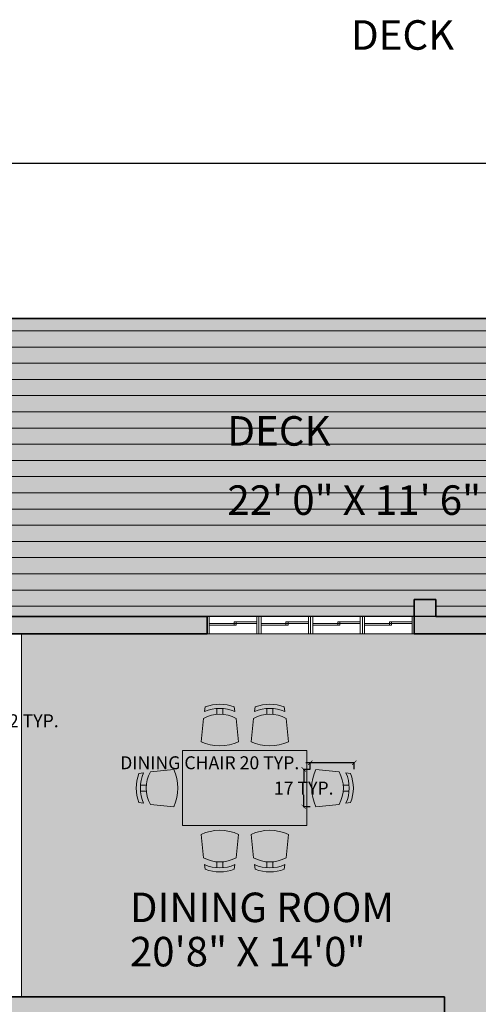
# Model space of a CAD drawing. Units: inches. Extents: x 1704 to 6393, y -157 to 1172.
# Tile 85 of 122: x 2081 to 2293, y 716 to 1172. Entities that reach past the tile are written whole.
import ezdxf

# ---------------------------------------------------------------- set-up
doc = ezdxf.new("R2010")
doc.units = ezdxf.units.IN
doc.header["$MEASUREMENT"] = 0
for name, color, linetype, lineweight in [('A-ANNO-DIMS', 7, 'Continuous', 13), ('A-AREA-IDEN', 7, 'Continuous', 18), ('A-FURN', 8, 'Continuous', 18), ('A-WALL-PATT', 7, 'Continuous', 13), ('C-PROP', 7, 'Continuous', 35), ('GLASS PANEL FASADE', 4, 'Continuous', 18), ('L-DECK-PLNK-PATT', 250, 'Continuous', 13), ('WALLS', 7, 'Continuous', 35)]:
    doc.layers.add(name, color=color, linetype=linetype, lineweight=lineweight)
for name, color, linetype, lineweight, true_color in [('A-FLOR-PATT', 7, 'Continuous', 13, 0xf2f2f2), ('A-FURN-PATT', 35, 'Continuous', 13, 0x8c775f), ('L-DECK-PATT', 35, 'Continuous', 13, 0xa6725b)]:
    doc.layers.add(name, color=color, linetype=linetype, lineweight=lineweight, true_color=true_color)
doc.styles.get("Standard").update_dxf_attribs({"font": 'arial.ttf'})
doc.dimstyles.get("Standard").update_dxf_attribs({"dimtxt": 6, "dimasz": 2, "dimexe": 0.18, "dimexo": 0.0625, "dimgap": 0.09, "dimtad": 0, "dimtih": 1, "dimtoh": 1, "dimdec": 1, "dimzin": 0, "dimdsep": 46, "dimlunit": 3, "dimtxsty": 'Standard', "dimblk": 'ARCHTICK', "dimcen": 0.09, "dimadec": 0, "dimazin": 0, "dimtfac": 1, "dimtdec": 1, "dimtofl": 0, "dimtmove": 0, "dimatfit": 3, "dimfxl": 1, "dimtolj": 1, "dimtzin": 0, "dimarcsym": 0})

# ---------------------------------------------------------------- blocks, each defined once
blk = doc.blocks.new('GLAZ-FOUR-PANEL-96')
for p, q in [((96, 8), (0, 8)), ((0, 8), (0, 0)), ((1, 8), (1, 0)), ((12.51, 4.77), (1, 4.77)), ((12.51, 4.77), (12.51, 5.55)), ((12.51, 5.55), (23, 5.55)), ((12.51, 4), (12.51, 4.77)), ((12.51, 4.77), (23, 4.77)), ((13.51, 4), (13.51, 5.55)), ((23, 8), (23, 0)), ((24, 8), (24, 0)), ((25, 8), (25, 0)), ((36.51, 4.77), (25, 4.77)), ((36.51, 4.77), (36.51, 5.55)), ((36.51, 5.55), (47, 5.55)), ((36.51, 4), (36.51, 4.77)), ((36.51, 4.77), (47, 4.77)), ((37.51, 4), (37.51, 5.55)), ((47, 8), (47, 0)), ((48, 8), (48, 0)), ((49, 8), (49, 0)), ((60.51, 4.77), (49, 4.77)), ((60.51, 4.77), (60.51, 5.55)), ((60.51, 5.55), (71, 5.55)), ((60.51, 4), (60.51, 4.77)), ((60.51, 4.77), (71, 4.77)), ((61.51, 4), (61.51, 5.55)), ((71, 8), (71, 0)), ((72, 8), (72, 0)), ((73, 8), (73, 0)), ((84.51, 4.77), (73, 4.77)), ((84.51, 4.77), (84.51, 5.55)), ((84.51, 5.55), (95, 5.55)), ((84.51, 4), (84.51, 4.77)), ((84.51, 4.77), (95, 4.77)), ((85.51, 4), (85.51, 5.55)), ((95, 0), (95, 8)), ((96, 0), (96, 8)), ((1, 4), (12.51, 4)), ((12.51, 4), (13.51, 4)), ((25, 4), (36.51, 4)), ((36.51, 4), (37.51, 4)), ((49, 4), (60.51, 4)), ((60.51, 4), (61.51, 4)), ((73, 4), (84.51, 4)), ((84.51, 4), (85.51, 4)), ((0, 0), (96, 0))]:
    blk.add_line(p, q)
blk = doc.blocks.new('CHAIR-DINING')
for p, q in [((3.42, 15.71), (1.25, 15.38)), ((17.36, 17.36), (6.56, 16.2)), ((1.98, 10.03), (4.69, 10.03)), ((1.98, 7.33), (4.69, 7.33)), ((3.42, 1.65), (1.25, 1.98)), ((17.36, 0), (6.56, 1.16))]:
    blk.add_line(p, q)
for centre, radius, start, end in [((18.51, 8.68), 18.51, 158.7887, 201.2113), ((19.31, 8.68), 17.38, 156.1344, 203.8656), ((20.26, 8.68), 15.63, 151.2372, 208.7628), ((-1.21, 8.68), 20.5, 334.9424, 25.0576)]:
    blk.add_arc(centre, radius, start, end)
blk = doc.blocks.new('_ArchTick')
at = {"color": 0, "linetype": 'ByBlock', "const_width": 0.15}
blk.add_lwpolyline([(-0.5, -0.5), (0.5, 0.5)], dxfattribs=at)
blk = doc.blocks.new('*D56')
at = {"layer": 'A-ANNO-DIMS', "color": 0, "lineweight": -2, "transparency": 16777216}
for p, q in [((2215.18, 827.57), (2213.18, 827.57)), ((2215.18, 824.58), (2215.18, 827.75)), ((2235.53, 827.57), (2215.18, 827.57)), ((2235.53, 824.58), (2235.53, 827.75))]:
    blk.add_line(p, q, dxfattribs=at)
at = {"layer": 'Defpoints', "color": 0, "lineweight": -3, "transparency": 16777216}
for p in [(2215.18, 827.57), (2215.18, 824.52), (2235.53, 824.52)]:
    blk.add_point(p, dxfattribs=at)
at = {"layer": 'A-ANNO-DIMS', "color": 0, "lineweight": -2, "transparency": 16777216, "xscale": 2, "yscale": 2, "zscale": 2, "rotation": 180}
blk.add_blockref('_ArchTick', (2215.18, 827.57), dxfattribs=at)
at = {"layer": 'A-ANNO-DIMS', "color": 0, "lineweight": -2, "transparency": 16777216, "xscale": 2, "yscale": 2, "zscale": 2}
blk.add_blockref('_ArchTick', (2235.53, 827.57), dxfattribs=at)
at = {"layer": 'A-ANNO-DIMS', "color": 0, "transparency": 16777216, "insert": (2168.6, 827.57), "char_height": 6, "attachment_point": 5}
blk.add_mtext('\\A1;DINING CHAIR 20 TYP.', dxfattribs=at)
blk = doc.blocks.new('*D57')
at = {"layer": 'A-ANNO-DIMS', "color": 0, "lineweight": -2, "transparency": 16777216}
for p, q in [((2215.12, 824.52), (2211.95, 824.52)), ((2212.13, 824.52), (2212.13, 818.94)), ((2212.13, 807.16), (2212.13, 812.73)), ((2215.12, 807.16), (2211.95, 807.16))]:
    blk.add_line(p, q, dxfattribs=at)
at = {"layer": 'Defpoints', "color": 0, "lineweight": -3, "transparency": 16777216}
for p in [(2215.18, 824.52), (2212.13, 807.16), (2215.18, 807.16)]:
    blk.add_point(p, dxfattribs=at)
at = {"layer": 'A-ANNO-DIMS', "color": 0, "lineweight": -2, "transparency": 16777216, "xscale": 2, "yscale": 2, "zscale": 2}
for p, rotation in [((2212.13, 824.52), 90), ((2212.13, 807.16), 270)]:
    blk.add_blockref('_ArchTick', p, dxfattribs=dict(at, rotation=rotation))
at = {"layer": 'A-ANNO-DIMS', "color": 0, "transparency": 16777216, "insert": (2212.13, 815.84), "char_height": 6, "attachment_point": 5}
blk.add_mtext('\\A1;17 TYP.', dxfattribs=at)
blk = doc.blocks.new('*D76')
at = {"layer": 'A-ANNO-DIMS', "color": 0, "lineweight": -2, "transparency": 16777216}
for p, q in [((2005.67, 851.74), (2005.67, 846.81)), ((2037.75, 851.74), (2037.75, 846.81)), ((2005.67, 846.99), (2037.75, 846.99)), ((2037.75, 846.99), (2039.75, 846.99))]:
    blk.add_line(p, q, dxfattribs=at)
at = {"layer": 'Defpoints', "color": 0, "lineweight": -3, "transparency": 16777216}
for p in [(2005.67, 851.81), (2037.75, 851.81), (2037.75, 846.99)]:
    blk.add_point(p, dxfattribs=at)
at = {"layer": 'A-ANNO-DIMS', "color": 0, "lineweight": -2, "transparency": 16777216, "xscale": 2, "yscale": 2, "zscale": 2, "rotation": 180}
blk.add_blockref('_ArchTick', (2005.67, 846.99), dxfattribs=at)
at = {"layer": 'A-ANNO-DIMS', "color": 0, "lineweight": -2, "transparency": 16777216, "xscale": 2, "yscale": 2, "zscale": 2}
blk.add_blockref('_ArchTick', (2037.75, 846.99), dxfattribs=at)
at = {"layer": 'A-ANNO-DIMS', "color": 0, "transparency": 16777216, "insert": (2070.27, 846.99), "char_height": 6, "attachment_point": 5}
blk.add_mtext('\\A1;SHRUB 32 TYP.', dxfattribs=at)
blk = doc.blocks.new('*D92')
at = {"layer": 'A-ANNO-DIMS', "color": 0, "lineweight": -2, "transparency": 16777216}
for p, q in [((2073.35, 895.28), (2073.35, 1105.29)), ((2073.35, 1105.11), (2332.66, 1105.11)), ((2605.35, 1105.11), (2346.04, 1105.11)), ((2605.35, 895.28), (2605.35, 1105.29))]:
    blk.add_line(p, q, dxfattribs=at)
at = {"layer": 'Defpoints', "color": 0, "lineweight": -3, "transparency": 16777216}
for p in [(2605.35, 1105.11), (2073.35, 895.21), (2605.35, 895.21)]:
    blk.add_point(p, dxfattribs=at)
at = {"layer": 'A-ANNO-DIMS', "color": 0, "lineweight": -2, "transparency": 16777216, "xscale": 2, "yscale": 2, "zscale": 2, "rotation": 180}
blk.add_blockref('_ArchTick', (2073.35, 1105.11), dxfattribs=at)
at = {"layer": 'A-ANNO-DIMS', "color": 0, "lineweight": -2, "transparency": 16777216, "xscale": 2, "yscale": 2, "zscale": 2}
blk.add_blockref('_ArchTick', (2605.35, 1105.11), dxfattribs=at)
at = {"layer": 'A-ANNO-DIMS', "color": 0, "transparency": 16777216, "insert": (2339.35, 1105.11), "char_height": 6, "attachment_point": 5}
blk.add_mtext('\\A1;532', dxfattribs=at)
blk = doc.blocks.new('*D93')
at = {"layer": 'A-ANNO-DIMS', "color": 0, "lineweight": -2, "transparency": 16777216}
for p, q in [((2605.29, 895.21), (1829.7, 895.21)), ((1829.88, 895.21), (1829.88, 495.87)), ((1829.88, 90.21), (1829.88, 489.56)), ((2605.29, 90.21), (1829.7, 90.21))]:
    blk.add_line(p, q, dxfattribs=at)
at = {"layer": 'Defpoints', "color": 0, "lineweight": -3, "transparency": 16777216}
for p in [(2605.35, 895.21), (1829.88, 90.21), (2605.35, 90.21)]:
    blk.add_point(p, dxfattribs=at)
at = {"layer": 'A-ANNO-DIMS', "color": 0, "lineweight": -2, "transparency": 16777216, "xscale": 2, "yscale": 2, "zscale": 2}
for p, rotation in [((1829.88, 895.21), 90), ((1829.88, 90.21), 270)]:
    blk.add_blockref('_ArchTick', p, dxfattribs=dict(at, rotation=rotation))
at = {"layer": 'A-ANNO-DIMS', "color": 0, "transparency": 16777216, "insert": (1829.88, 492.71), "char_height": 6, "attachment_point": 5}
blk.add_mtext('\\A1;805', dxfattribs=at)

msp = doc.modelspace()

# ---------------------------------------------------------------- hatches: boundary and pattern name
at = {"layer": 'A-FLOR-PATT', "transparency": 33554528}
h = msp.add_hatch(color=256, dxfattribs=at)
h.dxf.hatch_style = 1
h.paths.add_polyline_path([(2325.349, 863.213), (2325.349, 887.213), (2263.349, 887.213), (2167.349, 887.213), (2081.349, 887.213), (2081.349, 719.213), (2277.349, 719.213), (2277.349, 711.213), (2277.349, 372.213), (2349.349, 372.213), (2381.349, 372.213), (2381.349, 364.213), (2353.349, 364.213), (2353.349, 270.213), (2381.349, 270.213), (2381.349, 266.213), (2357.349, 266.213), (2357.349, 98.213), (2381.349, 98.213), (2385.181, 98.213), (2386.482, 98.213), (2424.215, 98.213), (2425.516, 98.213), (2429.349, 98.213), (2597.349, 98.213), (2597.349, 146.213), (2597.349, 218.213), (2597.349, 266.213), (2423.349, 266.213), (2423.349, 270.213), (2473.349, 270.213), (2473.349, 294.213), (2477.349, 294.213), (2477.349, 270.213), (2547.349, 270.213), (2547.349, 364.213), (2477.349, 364.213), (2477.349, 318.213), (2473.349, 318.213), (2473.349, 364.213), (2423.349, 364.213), (2423.349, 372.213), (2469.349, 372.213), (2469.349, 459.213), (2469.349, 538.213), (2350.349, 538.213), (2350.349, 565.713), (2358.349, 565.713), (2358.349, 545.213), (2420.349, 545.213), (2420.349, 610.213), (2358.349, 610.213), (2358.349, 589.713), (2350.349, 589.713), (2350.349, 615.213), (2425.349, 615.213), (2425.349, 607.213), (2425.349, 546.213), (2469.349, 546.213), (2514.349, 546.213), (2514.349, 607.213), (2449.349, 607.213), (2449.349, 615.213), (2451.738, 615.213), (2451.738, 659.213), (2427.738, 659.213), (2427.738, 665.213), (2367.738, 665.213), (2367.738, 667.213), (2367.738, 711.213), (2325.349, 711.213), (2325.349, 719.213), (2325.349, 755.213), (2325.349, 763.213)])
h.paths.add_polyline_path([(2233.858, 822.533, -0.187247), (2233.858, 809.14), (2231.697, 808.804, 0.0848928), (2233.131, 814.486), (2230.424, 814.486, -0.1042581), (2228.553, 808.313), (2217.751, 807.156, -0.2222222), (2217.751, 824.517), (2228.553, 823.359, -0.1042581), (2230.424, 817.186), (2233.131, 817.186, 0.0848928), (2231.697, 822.868)], flags=16)
h.paths.add_polyline_path([(2213.621, 833.197), (2213.621, 798.475), (2156.048, 798.475), (2156.048, 833.197)], flags=16)
h.paths.add_polyline_path([(2203.932, 848.099), (2205.089, 837.296, -0.2222222), (2187.728, 837.296), (2188.885, 848.099, -0.1042581), (2195.058, 849.969), (2195.058, 852.676, 0.0848928), (2189.377, 851.242), (2189.712, 853.404, -0.187247), (2203.105, 853.404), (2203.44, 851.242, 0.0848928), (2197.759, 852.676), (2197.759, 849.969, -0.1042581)], flags=16)
h.paths.add_polyline_path([(2181.941, 837.296, -0.2222222), (2164.58, 837.296), (2165.737, 848.099, -0.1042581), (2171.91, 849.969), (2171.91, 852.676, 0.0848928), (2166.229, 851.242), (2166.564, 853.404, -0.187247), (2179.957, 853.404), (2180.292, 851.242, 0.0848928), (2174.611, 852.676), (2174.611, 849.969, -0.1042581), (2180.784, 848.099)], flags=16)
h.paths.add_polyline_path([(2205.089, 794.376), (2203.932, 783.574, -0.1042581), (2197.759, 781.703), (2197.759, 778.996, 0.0848928), (2203.44, 780.43), (2203.105, 778.269, -0.187247), (2189.712, 778.269), (2189.377, 780.43, 0.0848928), (2195.058, 778.996), (2195.058, 781.703, -0.1042581), (2188.885, 783.574), (2187.728, 794.376, -0.2222222)], flags=16)
h.paths.add_polyline_path([(2181.941, 794.376), (2180.784, 783.574, -0.1042581), (2174.611, 781.703), (2174.611, 778.996, 0.0848928), (2180.292, 780.43), (2179.957, 778.269, -0.187247), (2166.564, 778.269), (2166.229, 780.43, 0.0848928), (2171.91, 778.996), (2171.91, 781.703, -0.1042581), (2165.737, 783.574), (2164.58, 794.376, -0.2222222)], flags=16)
h.paths.add_polyline_path([(2151.918, 807.156), (2141.116, 808.313, -0.1042581), (2139.245, 814.486), (2136.539, 814.486, 0.0848928), (2137.972, 808.804), (2135.811, 809.14, -0.187247), (2135.811, 822.533), (2137.972, 822.868, 0.0848928), (2136.539, 817.186), (2139.245, 817.186, -0.1042581), (2141.116, 823.359), (2151.918, 824.517, -0.2222222)], flags=16)
h.paths.add_polyline_path([(2357.868, 363.41), (2358.814, 363.41, 0.7537605)], flags=16)
h.paths.add_polyline_path([(2372.241, 363.117), (2372.248, 363.117), (2372.248, 363.343), (2371.302, 363.343), (2371.302, 363.139, -1.3603913)], flags=16)
h.paths.add_polyline_path([(2371.309, 272.716), (2371.302, 272.716), (2371.302, 272.49), (2372.248, 272.49), (2372.248, 272.693, -1.3603913)], flags=16)
h.paths.add_polyline_path([(2357.875, 272.716), (2357.868, 272.716), (2357.868, 272.49), (2358.814, 272.49), (2358.814, 272.693, -1.3603913)], flags=16)
h.paths.add_polyline_path([(2353.769, 363.074), (2376.347, 363.074), (2376.347, 272.759), (2353.769, 272.759)], flags=16)
h.paths.add_polyline_path([(2354.772, 362.07), (2375.344, 362.07), (2375.344, 273.762), (2354.772, 273.762)], flags=0)
h.paths.add_polyline_path([(2357.868, 363.343), (2358.814, 363.343), (2358.814, 363.117), (2357.868, 363.117)], flags=16)
h.paths.add_polyline_path([(2359.288, 359.184), (2359.288, 360.063), (2370.828, 360.063), (2370.828, 359.184), (2374.332, 359.184), (2374.332, 358.464), (2372.835, 358.464), (2372.835, 357.541), (2374.332, 357.541), (2374.332, 356.82), (2372.835, 356.82), (2372.835, 355.898), (2374.332, 355.898), (2374.332, 355.177), (2372.835, 355.177), (2372.835, 354.254), (2374.332, 354.254), (2374.332, 353.534), (2372.835, 353.534), (2372.835, 352.611), (2374.332, 352.611), (2374.332, 351.89), (2372.835, 351.89), (2372.835, 350.968), (2374.332, 350.968), (2374.332, 350.247), (2372.835, 350.247), (2372.835, 349.324), (2374.332, 349.324), (2374.332, 348.604), (2372.835, 348.604), (2372.835, 347.681), (2374.332, 347.681), (2374.332, 346.96), (2372.835, 346.96), (2372.835, 346.038), (2374.332, 346.038), (2374.332, 345.317), (2372.835, 345.317), (2372.835, 344.395), (2374.332, 344.395), (2374.332, 343.674), (2372.835, 343.674), (2372.835, 342.751), (2374.332, 342.751), (2374.332, 342.03), (2372.835, 342.03), (2372.835, 341.108), (2374.332, 341.108), (2374.332, 340.387), (2372.835, 340.387), (2372.835, 339.465), (2374.332, 339.465), (2374.332, 338.744), (2372.835, 338.744), (2372.835, 337.821), (2374.332, 337.821), (2374.332, 337.1), (2372.835, 337.1), (2372.835, 336.178), (2374.332, 336.178), (2374.332, 335.457), (2372.835, 335.457), (2372.835, 334.535), (2374.332, 334.535), (2374.332, 333.814), (2372.835, 333.814), (2372.835, 332.891), (2374.332, 332.891), (2374.332, 332.171), (2372.835, 332.171), (2372.835, 331.248), (2374.332, 331.248), (2374.332, 330.527), (2372.835, 330.527), (2372.835, 329.605), (2374.332, 329.605), (2374.332, 328.884), (2372.835, 328.884), (2372.835, 327.961), (2374.332, 327.961), (2374.332, 327.241), (2372.835, 327.241), (2372.835, 326.318), (2374.332, 326.318), (2374.332, 325.597), (2372.835, 325.597), (2372.835, 324.675), (2374.332, 324.675), (2374.332, 323.954), (2372.835, 323.954), (2372.835, 323.031), (2374.332, 323.031), (2374.332, 322.311), (2372.835, 322.311), (2372.835, 321.388), (2374.332, 321.388), (2374.332, 320.667), (2372.835, 320.667), (2372.835, 319.745), (2374.332, 319.745), (2374.332, 319.024), (2372.835, 319.024), (2372.835, 318.102), (2374.332, 318.102), (2374.332, 317.381), (2372.835, 317.381), (2372.835, 316.458), (2374.332, 316.458), (2374.332, 315.737), (2372.835, 315.737), (2372.835, 314.815), (2374.332, 314.815), (2374.332, 314.094), (2372.835, 314.094), (2372.835, 313.172), (2374.332, 313.172), (2374.332, 312.451), (2372.835, 312.451), (2372.835, 311.528), (2374.332, 311.528), (2374.332, 310.807), (2372.835, 310.807), (2372.835, 309.885), (2374.332, 309.885), (2374.332, 309.164), (2372.835, 309.164), (2372.835, 308.242), (2374.332, 308.242), (2374.332, 307.521), (2372.835, 307.521), (2372.835, 306.598), (2374.332, 306.598), (2374.332, 305.878), (2372.835, 305.878), (2372.835, 304.955), (2374.332, 304.955), (2374.332, 304.234), (2372.835, 304.234), (2372.835, 303.312), (2374.332, 303.312), (2374.332, 302.591), (2372.835, 302.591), (2372.835, 301.668), (2374.332, 301.668), (2374.332, 300.948), (2372.835, 300.948), (2372.835, 300.025), (2374.332, 300.025), (2374.332, 299.304), (2372.835, 299.304), (2372.835, 298.382), (2374.332, 298.382), (2374.332, 297.661), (2372.835, 297.661), (2372.835, 296.738), (2374.332, 296.738), (2374.332, 296.018), (2372.835, 296.018), (2372.835, 295.095), (2374.332, 295.095), (2374.332, 294.374), (2372.835, 294.374), (2372.835, 293.452), (2374.332, 293.452), (2374.332, 292.731), (2372.835, 292.731), (2372.835, 291.809), (2374.332, 291.809), (2374.332, 291.088), (2372.835, 291.088), (2372.835, 290.165), (2374.332, 290.165), (2374.332, 289.444), (2372.835, 289.444), (2372.835, 288.522), (2374.332, 288.522), (2374.332, 287.801), (2372.835, 287.801), (2372.835, 286.879), (2374.332, 286.879), (2374.332, 286.158), (2372.835, 286.158), (2372.835, 285.235), (2374.332, 285.235), (2374.332, 284.514), (2372.835, 284.514), (2372.835, 283.592), (2374.332, 283.592), (2374.332, 282.871), (2372.835, 282.871), (2372.835, 281.949), (2374.332, 281.949), (2374.332, 281.228), (2372.835, 281.228), (2372.835, 280.305), (2374.332, 280.305), (2374.332, 279.585), (2372.835, 279.585), (2372.835, 278.662), (2374.332, 278.662), (2374.332, 277.941), (2372.835, 277.941), (2372.835, 277.019), (2374.332, 277.019), (2374.332, 276.298), (2370.828, 276.298), (2370.828, 275.769), (2359.288, 275.769), (2359.288, 276.298), (2355.784, 276.298), (2355.784, 277.019), (2357.281, 277.019), (2357.281, 277.941), (2355.784, 277.941), (2355.784, 278.662), (2357.281, 278.662), (2357.281, 279.585), (2355.784, 279.585), (2355.784, 280.305), (2357.281, 280.305), (2357.281, 281.228), (2355.784, 281.228), (2355.784, 281.949), (2357.281, 281.949), (2357.281, 282.871), (2355.784, 282.871), (2355.784, 283.592), (2357.281, 283.592), (2357.281, 284.514), (2355.784, 284.514), (2355.784, 285.235), (2357.281, 285.235), (2357.281, 286.158), (2355.784, 286.158), (2355.784, 286.879), (2357.281, 286.879), (2357.281, 287.801), (2355.784, 287.801), (2355.784, 288.522), (2357.281, 288.522), (2357.281, 289.444), (2355.784, 289.444), (2355.784, 290.165), (2357.281, 290.165), (2357.281, 291.088), (2355.784, 291.088), (2355.784, 291.809), (2357.281, 291.809), (2357.281, 292.731), (2355.784, 292.731), (2355.784, 293.452), (2357.281, 293.452), (2357.281, 294.374), (2355.784, 294.374), (2355.784, 295.095), (2357.281, 295.095), (2357.281, 296.018), (2355.784, 296.018), (2355.784, 296.738), (2357.281, 296.738), (2357.281, 297.661), (2355.784, 297.661), (2355.784, 298.382), (2357.281, 298.382), (2357.281, 299.304), (2355.784, 299.304), (2355.784, 300.025), (2357.281, 300.025), (2357.281, 300.948), (2355.784, 300.948), (2355.784, 301.668), (2357.281, 301.668), (2357.281, 302.591), (2355.784, 302.591), (2355.784, 303.312), (2357.281, 303.312), (2357.281, 304.234), (2355.784, 304.234), (2355.784, 304.955), (2357.281, 304.955), (2357.281, 305.878), (2355.784, 305.878), (2355.784, 306.598), (2357.281, 306.598), (2357.281, 307.521), (2355.784, 307.521), (2355.784, 308.242), (2357.281, 308.242), (2357.281, 309.164), (2355.784, 309.164), (2355.784, 309.885), (2357.281, 309.885), (2357.281, 310.807), (2355.784, 310.807), (2355.784, 311.528), (2357.281, 311.528), (2357.281, 312.451), (2355.784, 312.451), (2355.784, 313.172), (2357.281, 313.172), (2357.281, 314.094), (2355.784, 314.094), (2355.784, 314.815), (2357.281, 314.815), (2357.281, 315.737), (2355.784, 315.737), (2355.784, 316.458), (2357.281, 316.458), (2357.281, 317.381), (2355.784, 317.381), (2355.784, 318.102), (2357.281, 318.102), (2357.281, 319.024), (2355.784, 319.024), (2355.784, 319.745), (2357.281, 319.745), (2357.281, 320.667), (2355.784, 320.667), (2355.784, 321.388), (2357.281, 321.388), (2357.281, 322.311), (2355.784, 322.311), (2355.784, 323.031), (2357.281, 323.031), (2357.281, 323.954), (2355.784, 323.954), (2355.784, 324.675), (2357.281, 324.675), (2357.281, 325.597), (2355.784, 325.597), (2355.784, 326.318), (2357.281, 326.318), (2357.281, 327.241), (2355.784, 327.241), (2355.784, 327.961), (2357.281, 327.961), (2357.281, 328.884), (2355.784, 328.884), (2355.784, 329.605), (2357.281, 329.605), (2357.281, 330.527), (2355.784, 330.527), (2355.784, 331.248), (2357.281, 331.248), (2357.281, 332.171), (2355.784, 332.171), (2355.784, 332.891), (2357.281, 332.891), (2357.281, 333.814), (2355.784, 333.814), (2355.784, 334.535), (2357.281, 334.535), (2357.281, 335.457), (2355.784, 335.457), (2355.784, 336.178), (2357.281, 336.178), (2357.281, 337.1), (2355.784, 337.1), (2355.784, 337.821), (2357.281, 337.821), (2357.281, 338.744), (2355.784, 338.744), (2355.784, 339.465), (2357.281, 339.465), (2357.281, 340.387), (2355.784, 340.387), (2355.784, 341.108), (2357.281, 341.108), (2357.281, 342.03), (2355.784, 342.03), (2355.784, 342.751), (2357.281, 342.751), (2357.281, 343.674), (2355.784, 343.674), (2355.784, 344.395), (2357.281, 344.395), (2357.281, 345.317), (2355.784, 345.317), (2355.784, 346.038), (2357.281, 346.038), (2357.281, 346.96), (2355.784, 346.96), (2355.784, 347.681), (2357.281, 347.681), (2357.281, 348.604), (2355.784, 348.604), (2355.784, 349.324), (2357.281, 349.324), (2357.281, 350.247), (2355.784, 350.247), (2355.784, 350.968), (2357.281, 350.968), (2357.281, 351.89), (2355.784, 351.89), (2355.784, 352.611), (2357.281, 352.611), (2357.281, 353.534), (2355.784, 353.534), (2355.784, 354.254), (2357.281, 354.254), (2357.281, 355.177), (2355.784, 355.177), (2355.784, 355.898), (2357.281, 355.898), (2357.281, 356.82), (2355.784, 356.82), (2355.784, 357.541), (2357.281, 357.541), (2357.281, 358.464), (2355.784, 358.464), (2355.784, 359.184)], flags=0)
at = {"layer": 'A-FURN-PATT'}
h = msp.add_hatch(color=256, dxfattribs=at)
h.dxf.hatch_style = 1
h.paths.add_polyline_path([(2151.918, 824.517), (2141.116, 823.359, 0.2564103), (2141.116, 808.313), (2151.918, 807.156, 0.2222222)])
h.paths.add_polyline_path([(2137.972, 822.868), (2135.811, 822.533, 0.187247), (2135.811, 809.14), (2137.972, 808.804, -0.2113308)])
h.paths.add_polyline_path([(2180.784, 848.099, 0.2564103), (2165.737, 848.099), (2164.58, 837.296, 0.2222222), (2181.941, 837.296)])
h.paths.add_polyline_path([(2179.957, 853.404, 0.187247), (2166.564, 853.404), (2166.229, 851.242, -0.2113308), (2180.292, 851.242)])
h.paths.add_polyline_path([(2174.611, 852.676, 0.0389066), (2171.91, 852.676), (2171.91, 849.969, -0.043264), (2174.611, 849.969)])
h.paths.add_polyline_path([(2203.932, 848.099, 0.2564103), (2188.885, 848.099), (2187.728, 837.296, 0.2222222), (2205.089, 837.296)])
h.paths.add_polyline_path([(2189.712, 853.404), (2189.377, 851.242, -0.2113308), (2203.44, 851.242), (2203.105, 853.404, 0.187247)])
h.paths.add_polyline_path([(2197.759, 852.676, 0.0389066), (2195.058, 852.676), (2195.058, 849.969, -0.043264), (2197.759, 849.969)])
h.paths.add_polyline_path([(2139.245, 817.186), (2136.539, 817.186, 0.0389066), (2136.539, 814.486), (2139.245, 814.486, -0.043264)])
h.paths.add_polyline_path([(2181.941, 794.376, 0.2222222), (2164.58, 794.376), (2165.737, 783.574, 0.2564103), (2180.784, 783.574)])
h.paths.add_polyline_path([(2174.611, 781.703, -0.043264), (2171.91, 781.703), (2171.91, 778.996, 0.0389066), (2174.611, 778.996)])
h.paths.add_polyline_path([(2180.292, 780.43, -0.2113308), (2166.229, 780.43), (2166.564, 778.269, 0.187247), (2179.957, 778.269)])
h.paths.add_polyline_path([(2205.089, 794.376, 0.2222222), (2187.728, 794.376), (2188.885, 783.574, 0.2564103), (2203.932, 783.574)])
h.paths.add_polyline_path([(2197.759, 781.703, -0.043264), (2195.058, 781.703), (2195.058, 778.996, 0.0389066), (2197.759, 778.996)])
h.paths.add_polyline_path([(2203.105, 778.269), (2203.44, 780.43, -0.2113308), (2189.377, 780.43), (2189.712, 778.269, 0.187247)])
h.paths.add_polyline_path([(2228.553, 823.359), (2217.751, 824.517, 0.2222222), (2217.751, 807.156), (2228.553, 808.313, 0.2564103)])
h.paths.add_polyline_path([(2233.131, 817.186), (2230.424, 817.186, -0.043264), (2230.424, 814.486), (2233.131, 814.486, 0.0389066)])
h.paths.add_polyline_path([(2233.858, 822.533), (2231.697, 822.868, -0.2113308), (2231.697, 808.804), (2233.858, 809.14, 0.187247)])
h = msp.add_hatch(color=256, dxfattribs=at)
h.dxf.hatch_style = 1
h.paths.add_polyline_path([(2213.621, 833.197), (2156.048, 833.197), (2156.048, 798.475), (2213.621, 798.475)])
at = {"layer": 'A-WALL-PATT', "transparency": 33554643}
h = msp.add_hatch(color=256, dxfattribs=at)
h.dxf.hatch_style = 1
h.paths.add_polyline_path([(2167.349, 895.213), (2073.349, 895.213), (2073.349, 887.213), (2081.349, 887.213), (2167.349, 887.213)])
h.paths.add_polyline_path([(2465.349, 895.213), (2273.349, 895.213), (2273.349, 903.213), (2263.349, 903.213), (2263.349, 895.213), (2263.349, 887.213), (2325.349, 887.213), (2325.349, 863.213), (2333.349, 863.213), (2333.349, 887.213), (2465.349, 887.213)])
h.paths.add_polyline_path([(2533.349, 895.213), (2513.349, 895.213), (2513.349, 887.213), (2513.349, 861.213), (2517.349, 861.213), (2517.349, 887.213), (2533.349, 887.213)])
h.paths.add_polyline_path([(2605.349, 895.213), (2581.349, 895.213), (2581.349, 887.213), (2597.349, 887.213), (2597.349, 854.213), (2605.349, 854.213)])
h.paths.add_polyline_path([(2605.349, 752.213), (2629.349, 752.213), (2629.349, 716.213), (2605.349, 716.213), (2605.349, 712.213), (2719.349, 712.213), (2719.349, 716.213), (2631.349, 716.213), (2631.349, 754.213), (2605.349, 754.213), (2605.349, 794.213), (2597.349, 794.213), (2597.349, 787.213), (2517.349, 787.213), (2517.349, 813.213), (2513.349, 813.213), (2513.349, 783.213), (2517.349, 783.213), (2597.349, 783.213), (2597.349, 719.213), (2517.349, 719.213), (2517.349, 753.213), (2513.349, 753.213), (2513.349, 719.213), (2365.349, 719.213), (2365.349, 763.213), (2325.349, 763.213), (2325.349, 755.213), (2357.349, 755.213), (2357.349, 719.213), (2325.349, 719.213), (2325.349, 711.213), (2547.349, 711.213), (2547.349, 615.213), (2449.349, 615.213), (2449.349, 607.213), (2514.349, 607.213), (2514.349, 546.213), (2439.349, 546.213), (2425.349, 546.213), (2425.349, 607.213), (2425.349, 615.213), (2350.349, 615.213), (2350.349, 589.713), (2358.349, 589.713), (2358.349, 610.213), (2420.349, 610.213), (2420.349, 545.213), (2358.349, 545.213), (2358.349, 565.713), (2350.349, 565.713), (2350.349, 538.213), (2469.349, 538.213), (2469.349, 459.213), (2469.349, 372.213), (2423.349, 372.213), (2423.349, 364.213), (2473.349, 364.213), (2473.349, 318.213), (2477.349, 318.213), (2477.349, 364.213), (2547.349, 364.213), (2547.349, 352.213), (2549.349, 352.213), (2549.349, 364.213), (2597.349, 364.213), (2597.349, 328.213), (2549.349, 328.213), (2547.349, 328.213), (2547.349, 326.213), (2549.349, 326.213), (2597.349, 326.213), (2605.349, 326.213), (2605.349, 377.057), (2597.349, 377.057), (2597.349, 372.213), (2477.349, 372.213), (2477.349, 451.213), (2597.349, 451.213), (2605.349, 451.213), (2605.349, 459.213), (2597.349, 459.213), (2477.349, 459.213), (2477.349, 538.213), (2597.349, 538.213), (2597.349, 495.213), (2605.349, 495.213), (2605.349, 512.213), (2631.349, 512.213), (2631.349, 568.213), (2605.349, 568.213), (2605.349, 577.213), (2597.349, 577.213), (2597.349, 542.213), (2518.349, 542.213), (2518.349, 607.213), (2532.349, 607.213), (2605.349, 607.213), (2605.349, 615.213), (2597.349, 615.213), (2551.349, 615.213), (2551.349, 711.213), (2597.349, 711.213), (2597.349, 645.213), (2605.349, 645.213), (2605.349, 712.213), (2605.349, 716.213)])
h.paths.add_polyline_path([(2605.349, 566.213), (2629.349, 566.213), (2629.349, 514.213), (2605.349, 514.213)], flags=16)
h.paths.add_polyline_path([(2381.349, 372.213), (2349.349, 372.213), (2349.349, 202.213), (2337.349, 202.213), (2337.349, 194.213), (2349.349, 194.213), (2349.349, 90.213), (2349.349, 72.213), (2357.349, 72.213), (2357.349, 90.213), (2381.349, 90.213), (2381.349, 98.213), (2357.349, 98.213), (2357.349, 266.213), (2381.349, 266.213), (2381.349, 270.213), (2353.349, 270.213), (2353.349, 364.213), (2381.349, 364.213)])
h.paths.add_polyline_path([(2605.349, 302.213), (2597.349, 302.213), (2597.349, 270.213), (2477.349, 270.213), (2477.349, 294.213), (2473.349, 294.213), (2473.349, 270.213), (2423.349, 270.213), (2423.349, 266.213), (2597.349, 266.213), (2597.349, 218.213), (2605.349, 218.213)])
h.paths.add_polyline_path([(2605.349, 146.213), (2597.349, 146.213), (2597.349, 98.213), (2429.349, 98.213), (2429.349, 90.213), (2597.349, 90.213), (2597.349, 72.213), (2605.349, 72.213), (2605.349, 90.213)])
h.paths.add_polyline_path([(2225.349, 202.213), (2049.349, 202.213), (2049.349, 194.213), (2225.349, 194.213)])
h.paths.add_polyline_path([(2289.349, 202.213), (2277.349, 202.213), (2273.349, 202.213), (2269.516, 202.213), (2269.516, 194.213), (2273.349, 194.213), (2277.349, 194.213), (2289.349, 194.213)])
h.paths.add_polyline_path([(2273.349, 372.213), (2029.19, 372.213), (2029.19, 364.213), (2273.349, 364.213)])
h.paths.add_polyline_path([(2277.349, 545.213), (2213.349, 545.213), (2213.349, 573.213), (2205.349, 573.213), (2177.349, 573.213), (2177.349, 545.213), (2073.349, 545.213), (2073.349, 538.213), (2081.349, 538.213), (2277.349, 538.213)])
h.paths.add_polyline_path([(2181.349, 545.213), (2181.349, 569.213), (2205.349, 569.213), (2205.349, 545.213)], flags=16)
h.paths.add_polyline_path([(2277.349, 719.213), (2081.349, 719.213), (2073.349, 719.213), (2073.349, 711.213), (2154.575, 711.213), (2205.349, 711.213), (2205.349, 687.213), (2205.349, 629.213), (2213.349, 629.213), (2273.349, 629.213), (2273.349, 631.213), (2207.349, 631.213), (2207.349, 707.213), (2231.349, 707.213), (2231.349, 709.213), (2207.349, 709.213), (2207.349, 711.213), (2277.349, 711.213)])
at = {"layer": 'L-DECK-PATT', "transparency": 33554544}
h = msp.add_hatch(color=256, dxfattribs=at)
h.dxf.hatch_style = 1
h.paths.add_polyline_path([(2329.589, 1033.213), (2065.589, 1033.213), (2065.589, 895.213), (2167.349, 895.213), (2263.349, 895.213), (2263.349, 903.213), (2273.349, 903.213), (2273.349, 895.213), (2329.589, 895.213)])
h.paths.add_polyline_path([(2664.349, 1033.213), (2333.589, 1033.213), (2333.589, 895.213), (2465.349, 895.213), (2469.181, 895.213), (2470.482, 895.213), (2508.215, 895.213), (2509.516, 895.213), (2513.349, 895.213), (2533.349, 895.213), (2581.349, 895.213), (2605.349, 895.213), (2664.349, 895.213)])
h.paths.add_polyline_path([(2333.589, 1033.213), (2329.589, 1033.213), (2329.589, 895.213), (2333.589, 895.213)])
at = {"layer": 'L-DECK-PLNK-PATT'}
h = msp.add_hatch(dxfattribs=at)
h.set_pattern_fill('LINE', color=256, scale=60)
h.paths.add_polyline_path([(2329.589, 1033.213), (2065.589, 1033.213), (2065.589, 895.213), (2167.349, 895.213), (2263.349, 895.213), (2263.349, 903.213), (2273.349, 903.213), (2273.349, 895.213), (2329.589, 895.213)])
h.paths.add_polyline_path([(2664.349, 1033.213), (2333.589, 1033.213), (2333.589, 895.213), (2465.349, 895.213), (2469.181, 895.213), (2470.482, 895.213), (2508.215, 895.213), (2509.516, 895.213), (2513.349, 895.213), (2533.349, 895.213), (2581.349, 895.213), (2605.349, 895.213), (2664.349, 895.213)])
h.paths.add_polyline_path([(2333.589, 1033.213), (2329.589, 1033.213), (2329.589, 895.213), (2333.589, 895.213)])

# ---------------------------------------------------------------- linework, layer by layer
at = {"layer": 'A-FURN'}
for p, q in [((2156.048, 833.197), (2156.048, 798.475)), ((2156.048, 833.197), (2213.621, 833.197)), ((2213.621, 833.197), (2213.621, 798.475)), ((2156.048, 798.475), (2213.621, 798.475))]:
    msp.add_line(p, q, dxfattribs=at)
at = {"layer": 'C-PROP'}
msp.add_line((2723.349, 1033.213), (1898.349, 1033.213), dxfattribs=at)
at = {"layer": 'GLASS PANEL FASADE'}
msp.add_lwpolyline([(2081.349, 719.213), (2073.349, 719.213), (2073.349, 887.213), (2081.349, 887.213)], close=True, dxfattribs=at)
at = {"layer": 'WALLS'}
for p, q in [((2263.349, 895.213), (2263.349, 903.213)), ((2263.349, 903.213), (2273.349, 903.213)), ((2273.349, 903.213), (2273.349, 895.213)), ((2167.349, 895.213), (1898.349, 895.213)), ((2167.349, 887.213), (2167.349, 895.213)), ((2263.349, 887.213), (2263.349, 895.213)), ((2465.349, 895.213), (2273.349, 895.213)), ((2081.349, 887.213), (2073.349, 887.213)), ((2167.349, 887.213), (2081.349, 887.213)), ((2325.349, 887.213), (2263.349, 887.213)), ((2081.349, 719.213), (2073.349, 719.213)), ((2277.349, 719.213), (2081.349, 719.213)), ((2277.349, 719.213), (2277.349, 711.213))]:
    msp.add_line(p, q, dxfattribs=at)

# ---------------------------------------------------------------- block references
at = {"layer": 'A-FURN'}
for p, rotation in [((2164.58, 854.657), 269.9999999999997), ((2187.729, 854.657), 269.9999999999986), ((2235.112, 824.516), 180), ((2181.941, 777.015), 90.0000000000037), ((2205.089, 777.015), 90.00000000000152)]:
    msp.add_blockref('CHAIR-DINING', p, dxfattribs=dict(at, rotation=rotation))
msp.add_blockref('CHAIR-DINING', (2134.557, 807.156), dxfattribs=at)
at = {"layer": 'GLASS PANEL FASADE'}
msp.add_blockref('GLAZ-FOUR-PANEL-96', (2167.349, 887.213), dxfattribs=at)

# ---------------------------------------------------------------- texts
at = {"layer": 'A-ANNO-DIMS'}
for s, p in [('22\' 0" X 11\' 6"', (2176.783, 942.309)), ('20\'8" X 14\'0"', (2131.612, 733.314))]:
    msp.add_text(s, height=13.6672, dxfattribs=at).set_placement(p)
at = {"layer": 'A-AREA-IDEN'}
for s, p in [('DECK', (2234.042, 1157.602)), ('DECK', (2176.783, 974.341)), ('DINING ROOM', (2131.612, 753.797))]:
    msp.add_text(s, height=13.6672, dxfattribs=at).set_placement(p)

# ---------------------------------------------------------------- dimensions: what is measured, and where the dimension line sits
at = {"layer": 'A-ANNO-DIMS'}
dim = msp.add_linear_dim(base=(2605.349, 1105.107), p1=(2073.349, 895.213), p2=(2605.349, 895.213), dimstyle='Standard', override={"dimdec": 0, "dimlfac": 1, "dimrnd": 0, "dimzin": 0, "dimdsep": 46, "dimlunit": 2}, dxfattribs=at)
dim.commit()
dim.dimension.update_dxf_attribs({"geometry": '*D92', "text_midpoint": (2339.349, 1105.107)})
dim = msp.add_linear_dim(base=(1829.878, 90.213), p1=(2605.349, 895.213), p2=(2605.349, 90.213), angle=90, dimstyle='Standard', override={"dimdec": 0, "dimlfac": 1, "dimrnd": 0, "dimzin": 0, "dimdsep": 46, "dimlunit": 2}, dxfattribs=at)
dim.commit()
dim.dimension.update_dxf_attribs({"geometry": '*D93', "text_midpoint": (1829.878, 492.713)})
dim = msp.add_linear_dim(base=(2037.753, 846.993), p1=(2005.67, 851.806), p2=(2037.753, 851.806), text='SHRUB <> TYP.', dimstyle='Standard', override={"dimdec": 0, "dimlfac": 1, "dimrnd": 0, "dimzin": 0, "dimdsep": 46, "dimlunit": 2}, dxfattribs=at)
dim.commit()
dim.dimension.update_dxf_attribs({"geometry": '*D76', "text_midpoint": (2070.267, 846.993)})
for base, p1, p2, angle, text, picture, middle in [((2215.179, 827.569), (2235.53, 824.517), (2215.179, 824.517), 180, 'DINING CHAIR <> TYP.', '*D56', (2168.598, 827.569)), ((2212.126, 807.156), (2215.179, 824.517), (2215.179, 807.156), 270, '<> TYP.', '*D57', (2212.126, 815.836))]:
    dim = msp.add_linear_dim(base=base, p1=p1, p2=p2, angle=angle, text=text, dimstyle='Standard', override={"dimdec": 0, "dimlfac": 1, "dimrnd": 0, "dimzin": 0, "dimdsep": 46, "dimlunit": 2}, dxfattribs=at)
    dim.commit()
    dim.dimension.update_dxf_attribs({"geometry": picture, "text_midpoint": middle})

doc.saveas('drawing.dxf')
